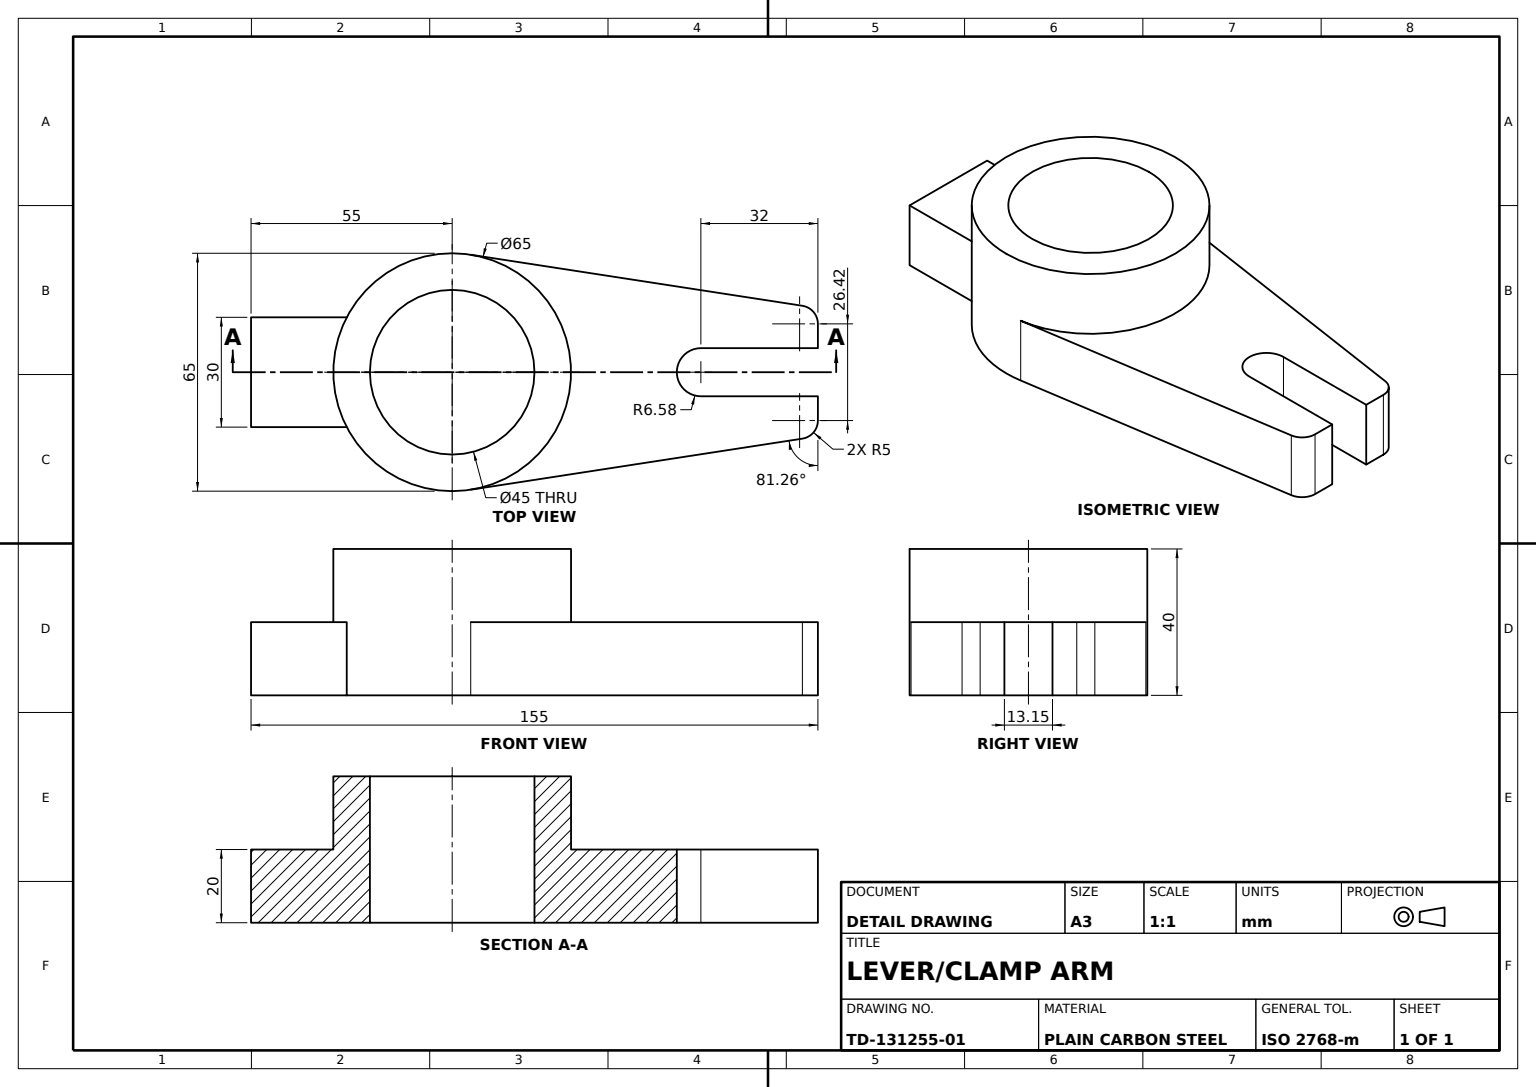
from build123d import *

# Parameters (mm, degrees)
HUB_PROFILE_65_45_R   = 32.5
HUB_PROFILE_65_45_R_2 = 22.5
HUB_65_BORE_45_DEPTH  = 40
FORK_ARM_DEPTH        = 20
REAR_BLOCK_DEPTH      = 20


with BuildPart() as part:
    # Hub Profile Ø65-Ø45 → Hub Ø65 Bore Ø45 (new body)
    with BuildSketch(Plane(origin=(0, 0, 0), x_dir=(1, 0, 0), z_dir=(0, 1, 0))):
        with Locations(Location((0, 0, 0), (0, 0, 270))):
            Circle(HUB_PROFILE_65_45_R)
        with Locations(Location((0, 0, 0), (0, 0, 270))):
            Circle(HUB_PROFILE_65_45_R_2, mode=Mode.SUBTRACT)
    extrude(amount=HUB_65_BORE_45_DEPTH)

    # Fork Arm Profile → Fork Arm (add)
    with BuildSketch(Plane(origin=(0, 0, 0), x_dir=(1, 0, 0), z_dir=(0, 1, 0))):
        with BuildLine():
            Line((68, 6.576589216), (100, 6.576589216))
            Line((100, 6.576589216), (100, 13.210293464))
            ThreePointArc((100, 13.210293464), (98.79478546, 16.465996662), (95.760158675, 18.152171527))
            Line((95.760158675, 18.152171527), (5.067811416, 32.102449867))
            ThreePointArc((5.067811416, 32.102449867), (32.5, 0), (5.067811416, -32.102449867))
            Line((5.067811416, -32.102449867), (95.760158675, -18.152171527))
            ThreePointArc((95.760158675, -18.152171527), (98.79478546, -16.465996662), (100, -13.210293464))
            Line((100, -13.210293464), (100, -6.576589216))
            Line((100, -6.576589216), (68, -6.576589216))
            ThreePointArc((68, -6.576589216), (61.423410784, 0), (68, 6.576589216))
        make_face()
    extrude(amount=FORK_ARM_DEPTH)

    # Rear Block Profile 30x55 → Rear Block (add)
    with BuildSketch(Plane(origin=(0, 0, 0), x_dir=(1, 0, 0), z_dir=(0, 1, 0))):
        with BuildLine():
            Line((-55, -15), (-55, 15))
            Line((-55, 15), (-28.831406487, 15))
            ThreePointArc((-28.831406487, 15), (-32.5, 0), (-28.831406487, -15))
            Line((-28.831406487, -15), (-55, -15))
        make_face()
    extrude(amount=REAR_BLOCK_DEPTH)


solid = part.part
